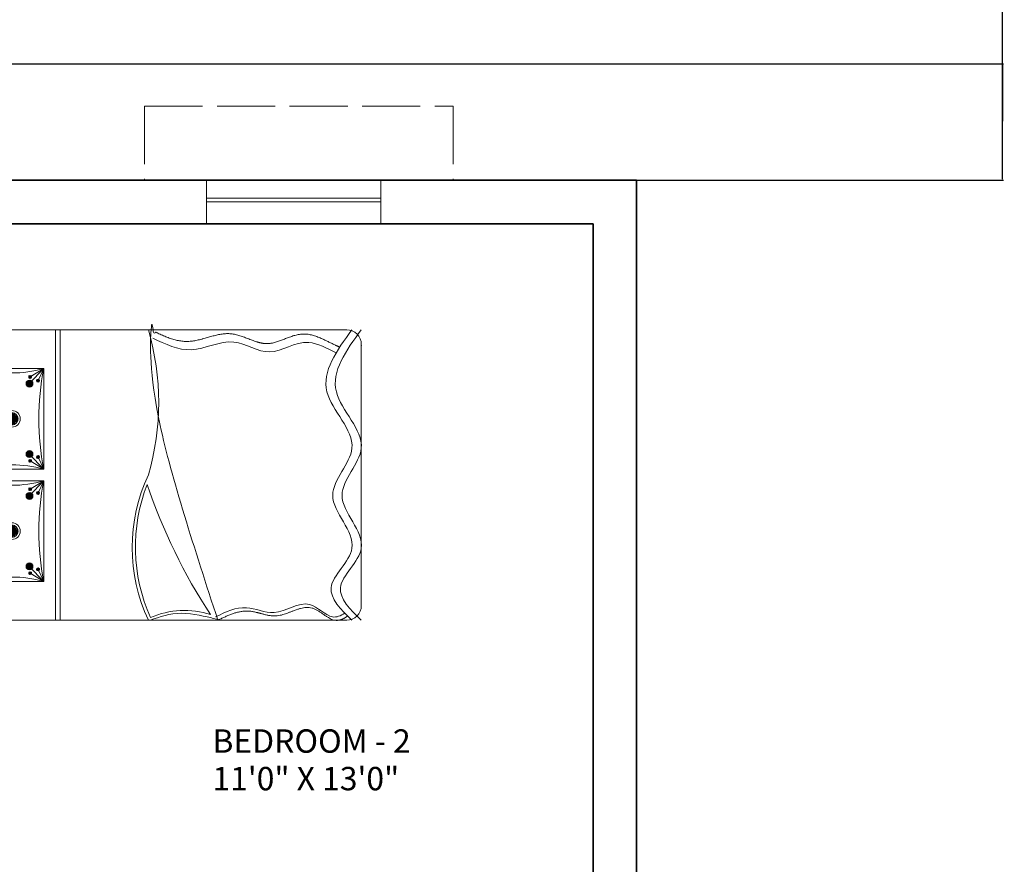
# Model space of a CAD drawing. Units: inches. Extents: x -61 to 1599, y -1316 to 257.
# Tile 182 of 204: x 1395 to 1599, y -753 to -579. Entities that reach past the tile are written whole.
import ezdxf

# ---------------------------------------------------------------- set-up
doc = ezdxf.new("R2010")
doc.units = ezdxf.units.IN
doc.header["$MEASUREMENT"] = 0
doc.linetypes.add('ACAD_ISO02W100', pattern=[15, 12, -3])
for name, color, linetype, lineweight in [('A-ANNO-DIMS', 2, 'Continuous', 18), ('A-AREA-IDEN', 1, 'Continuous', 18), ('A-FLOR-OVHD', 203, 'ACAD_ISO02W100', 13), ('FURNITURE', 83, 'Continuous', 18), ('WALLS', 4, 'Continuous', 35), ('WINDOWS', 220, 'Continuous', 18)]:
    doc.layers.add(name, color=color, linetype=linetype, lineweight=lineweight)
doc.layers.add('LT', color=8, linetype='Continuous')
doc.styles.get("Standard").update_dxf_attribs({"font": 'arial.ttf'})
doc.dimstyles.get("Standard").update_dxf_attribs({"dimtxt": 0.18, "dimasz": 0.18, "dimexe": 0.18, "dimexo": 0.0625, "dimgap": 0.09, "dimtad": 0, "dimtih": 1, "dimtoh": 1, "dimdec": 0, "dimzin": 0, "dimdsep": 46, "dimlunit": 3, "dimtxsty": 'Standard', "dimcen": 0.09, "dimadec": 0, "dimazin": 0, "dimtfac": 1, "dimtdec": 0, "dimtofl": 0, "dimtmove": 0, "dimatfit": 3, "dimfxl": 1, "dimtolj": 1, "dimtzin": 0, "dimarcsym": 0})

# ---------------------------------------------------------------- blocks, each defined once
blk = doc.blocks.new('WIN-36IN')
for p, q in [((0, 4.5), (0, 9)), ((0, 9), (0, 0)), ((36, 9), (36, 0)), ((0, 5.26), (36, 5.26)), ((0, 4.5), (36, 4.5)), ((0, 4.5), (36, 4.5))]:
    blk.add_line(p, q)
blk = doc.blocks.new('*U100')
at = {"layer": 'LT'}
blk.add_line((0, 0.15), (0, -0.15), dxfattribs=at)
for centre, start, end in [((0.44, 0), 160.9983, 199.0017), ((-0.44, 0), 340.9983, 19.0017)]:
    blk.add_arc(centre, 0.468, start, end, dxfattribs=at)
blk = doc.blocks.new('*U101')
at = {"layer": 'LT', "transparency": 16777216}
for p, rotation in [((-57.96, -16.31), 72), ((-57.93, -16.26), 48.00000000000001), ((-57.87, -16.22), 24), ((-57.75, -16.22), 336), ((-57.7, -16.26), 312), ((-57.67, -16.31), 288), ((-57.96, -16.37), 96), ((-57.94, -16.43), 120), ((-57.9, -16.48), 144), ((-57.84, -16.51), 168.0000000000001), ((-57.78, -16.51), 192), ((-57.72, -16.48), 216), ((-57.68, -16.43), 240), ((-57.66, -16.37), 264)]:
    blk.add_blockref('*U100', p, dxfattribs=dict(at, rotation=rotation))
blk.add_blockref('*U100', (-57.81, -16.21), dxfattribs=at)
blk = doc.blocks.new('*U104')
at = {"layer": 'LT'}
blk.add_line((0, 0.15), (0, -0.15), dxfattribs=at)
for centre, start, end in [((0.44, 0), 160.9983, 199.0017), ((-0.44, 0), 340.9983, 19.0017)]:
    blk.add_arc(centre, 0.468, start, end, dxfattribs=at)
blk = doc.blocks.new('*U105')
at = {"layer": 'LT', "transparency": 16777216}
for p, rotation in [((-57.96, -16.31), 72), ((-57.93, -16.26), 48.00000000000001), ((-57.87, -16.22), 24), ((-57.75, -16.22), 336), ((-57.7, -16.26), 312), ((-57.67, -16.31), 288), ((-57.96, -16.37), 96), ((-57.94, -16.43), 120), ((-57.9, -16.48), 144), ((-57.84, -16.51), 168.0000000000001), ((-57.78, -16.51), 192), ((-57.72, -16.48), 216), ((-57.68, -16.43), 240), ((-57.66, -16.37), 264)]:
    blk.add_blockref('*U104', p, dxfattribs=dict(at, rotation=rotation))
blk.add_blockref('*U104', (-57.81, -16.21), dxfattribs=at)
blk = doc.blocks.new('*U71')
at = {"layer": 'LT'}
blk.add_line((0, 0.15), (0, -0.15), dxfattribs=at)
for centre, start, end in [((0.44, 0), 160.9983, 199.0017), ((-0.44, 0), 340.9983, 19.0017)]:
    blk.add_arc(centre, 0.468, start, end, dxfattribs=at)
blk = doc.blocks.new('*U58')
at = {"layer": 'LT', "transparency": 16777216}
for p, rotation in [((-57.96, -16.31), 72), ((-57.93, -16.26), 48.00000000000001), ((-57.87, -16.22), 24), ((-57.75, -16.22), 336), ((-57.7, -16.26), 312), ((-57.67, -16.31), 288), ((-57.96, -16.37), 96), ((-57.94, -16.43), 120), ((-57.9, -16.48), 144), ((-57.84, -16.51), 168.0000000000001), ((-57.78, -16.51), 192), ((-57.72, -16.48), 216), ((-57.68, -16.43), 240), ((-57.66, -16.37), 264)]:
    blk.add_blockref('*U71', p, dxfattribs=dict(at, rotation=rotation))
blk.add_blockref('*U71', (-57.81, -16.21), dxfattribs=at)
blk = doc.blocks.new('*U61')
at = {"layer": 'LT'}
blk.add_line((0, 0.15), (0, -0.15), dxfattribs=at)
for centre, start, end in [((0.44, 0), 160.9983, 199.0017), ((-0.44, 0), 340.9983, 19.0017)]:
    blk.add_arc(centre, 0.468, start, end, dxfattribs=at)
blk = doc.blocks.new('*U62')
at = {"layer": 'LT', "transparency": 16777216}
for p, rotation in [((-57.96, -16.31), 72), ((-57.93, -16.26), 48.00000000000001), ((-57.87, -16.22), 24), ((-57.75, -16.22), 336), ((-57.7, -16.26), 312), ((-57.67, -16.31), 288), ((-57.96, -16.37), 96), ((-57.94, -16.43), 120), ((-57.9, -16.48), 144), ((-57.84, -16.51), 168.0000000000001), ((-57.78, -16.51), 192), ((-57.72, -16.48), 216), ((-57.68, -16.43), 240), ((-57.66, -16.37), 264)]:
    blk.add_blockref('*U61', p, dxfattribs=dict(at, rotation=rotation))
blk.add_blockref('*U61', (-57.81, -16.21), dxfattribs=at)
blk = doc.blocks.new('*U94')
at = {"layer": 'LT'}
blk.add_line((0, 0.36), (0, -0.36), dxfattribs=at)
for centre, start, end in [((1.04, 0), 160.9983, 199.0017), ((-1.04, 0), 340.9983, 19.0017)]:
    blk.add_arc(centre, 1.1, start, end, dxfattribs=at)
blk = doc.blocks.new('*U95')
at = {"layer": 'LT', "transparency": 16777216}
for p, rotation in [((-136.32, -38.51), 96), ((-136.3, -38.36), 72), ((-136.27, -38.65), 120), ((-136.23, -38.23), 48.00000000000001), ((-136.17, -38.76), 144), ((-136.11, -38.14), 23.99999999999999), ((-136.04, -38.82), 168.0000000000001), ((-135.82, -38.14), 336.0000000000001), ((-135.89, -38.82), 191.9999999999999), ((-135.75, -38.76), 216), ((-135.69, -38.23), 312), ((-135.65, -38.65), 240), ((-135.62, -38.36), 288.0000000000001), ((-135.6, -38.51), 264)]:
    blk.add_blockref('*U94', p, dxfattribs=dict(at, rotation=rotation))
blk.add_blockref('*U94', (-135.96, -38.11), dxfattribs=at)
blk = doc.blocks.new('*U57')
at = {"layer": 'LT'}
blk.add_line((0, 0.36), (0, -0.36), dxfattribs=at)
for centre, start, end in [((1.04, 0), 160.9983, 199.0017), ((-1.04, 0), 340.9983, 19.0017)]:
    blk.add_arc(centre, 1.1, start, end, dxfattribs=at)
blk = doc.blocks.new('*U99')
at = {"layer": 'LT', "transparency": 16777216}
for p, rotation in [((-136.32, -38.51), 96), ((-136.3, -38.36), 72), ((-136.27, -38.65), 120), ((-136.23, -38.23), 48.00000000000001), ((-136.17, -38.76), 144), ((-136.11, -38.14), 23.99999999999999), ((-136.04, -38.82), 168.0000000000001), ((-135.82, -38.14), 336.0000000000001), ((-135.89, -38.82), 191.9999999999999), ((-135.75, -38.76), 216), ((-135.69, -38.23), 312), ((-135.65, -38.65), 240), ((-135.62, -38.36), 288.0000000000001), ((-135.6, -38.51), 264)]:
    blk.add_blockref('*U57', p, dxfattribs=dict(at, rotation=rotation))
blk.add_blockref('*U57', (-135.96, -38.11), dxfattribs=at)
blk = doc.blocks.new('*U80')
at = {"layer": 'LT'}
blk.add_line((0, 0.36), (0, -0.36), dxfattribs=at)
for centre, start, end in [((1.04, 0), 160.9983, 199.0017), ((-1.04, 0), 340.9983, 19.0017)]:
    blk.add_arc(centre, 1.1, start, end, dxfattribs=at)
blk = doc.blocks.new('*U96')
at = {"layer": 'LT', "transparency": 16777216}
for p, rotation in [((-136.32, -38.51), 96), ((-136.3, -38.36), 72), ((-136.27, -38.65), 120), ((-136.23, -38.23), 48.00000000000001), ((-136.17, -38.76), 144), ((-136.11, -38.14), 23.99999999999999), ((-136.04, -38.82), 168.0000000000001), ((-135.82, -38.14), 336.0000000000001), ((-135.89, -38.82), 191.9999999999999), ((-135.75, -38.76), 216), ((-135.69, -38.23), 312), ((-135.65, -38.65), 240), ((-135.62, -38.36), 288.0000000000001), ((-135.6, -38.51), 264)]:
    blk.add_blockref('*U80', p, dxfattribs=dict(at, rotation=rotation))
blk.add_blockref('*U80', (-135.96, -38.11), dxfattribs=at)
blk = doc.blocks.new('*U69')
at = {"layer": 'LT'}
blk.add_line((0, 0.36), (0, -0.36), dxfattribs=at)
for centre, start, end in [((1.04, 0), 160.9983, 199.0017), ((-1.04, 0), 340.9983, 19.0017)]:
    blk.add_arc(centre, 1.1, start, end, dxfattribs=at)
blk = doc.blocks.new('*U70')
at = {"layer": 'LT', "transparency": 16777216}
for p, rotation in [((-136.32, -38.51), 96), ((-136.3, -38.36), 72), ((-136.27, -38.65), 120), ((-136.23, -38.23), 48.00000000000001), ((-136.17, -38.76), 144), ((-136.11, -38.14), 23.99999999999999), ((-136.04, -38.82), 168.0000000000001), ((-135.82, -38.14), 336.0000000000001), ((-135.89, -38.82), 191.9999999999999), ((-135.75, -38.76), 216), ((-135.69, -38.23), 312), ((-135.65, -38.65), 240), ((-135.62, -38.36), 288.0000000000001), ((-135.6, -38.51), 264)]:
    blk.add_blockref('*U69', p, dxfattribs=dict(at, rotation=rotation))
blk.add_blockref('*U69', (-135.96, -38.11), dxfattribs=at)
blk = doc.blocks.new('*U102')
at = {"layer": 'LT'}
blk.add_line((0, 0.15), (0, -0.15), dxfattribs=at)
for centre, start, end in [((0.44, 0), 160.9983, 199.0017), ((-0.44, 0), 340.9983, 19.0017)]:
    blk.add_arc(centre, 0.468, start, end, dxfattribs=at)
blk = doc.blocks.new('*U103')
at = {"layer": 'LT', "transparency": 16777216}
for p, rotation in [((-57.96, -16.31), 72), ((-57.93, -16.26), 48.00000000000001), ((-57.87, -16.22), 24), ((-57.75, -16.22), 336), ((-57.7, -16.26), 312), ((-57.67, -16.31), 288), ((-57.96, -16.37), 96), ((-57.94, -16.43), 120), ((-57.9, -16.48), 144), ((-57.84, -16.51), 168.0000000000001), ((-57.78, -16.51), 192), ((-57.72, -16.48), 216), ((-57.68, -16.43), 240), ((-57.66, -16.37), 264)]:
    blk.add_blockref('*U102', p, dxfattribs=dict(at, rotation=rotation))
blk.add_blockref('*U102', (-57.81, -16.21), dxfattribs=at)
blk = doc.blocks.new('*U55')
at = {"layer": 'LT'}
blk.add_line((0, 0.15), (0, -0.15), dxfattribs=at)
for centre, start, end in [((0.44, 0), 160.9983, 199.0017), ((-0.44, 0), 340.9983, 19.0017)]:
    blk.add_arc(centre, 0.468, start, end, dxfattribs=at)
blk = doc.blocks.new('*U56')
at = {"layer": 'LT', "transparency": 16777216}
for p, rotation in [((-57.96, -16.31), 72), ((-57.93, -16.26), 48.00000000000001), ((-57.87, -16.22), 24), ((-57.75, -16.22), 336), ((-57.7, -16.26), 312), ((-57.67, -16.31), 288), ((-57.96, -16.37), 96), ((-57.94, -16.43), 120), ((-57.9, -16.48), 144), ((-57.84, -16.51), 168.0000000000001), ((-57.78, -16.51), 192), ((-57.72, -16.48), 216), ((-57.68, -16.43), 240), ((-57.66, -16.37), 264)]:
    blk.add_blockref('*U55', p, dxfattribs=dict(at, rotation=rotation))
blk.add_blockref('*U55', (-57.81, -16.21), dxfattribs=at)
blk = doc.blocks.new('*U59')
at = {"layer": 'LT'}
blk.add_line((0, 0.15), (0, -0.15), dxfattribs=at)
for centre, start, end in [((0.44, 0), 160.9983, 199.0017), ((-0.44, 0), 340.9983, 19.0017)]:
    blk.add_arc(centre, 0.468, start, end, dxfattribs=at)
blk = doc.blocks.new('*U60')
at = {"layer": 'LT', "transparency": 16777216}
for p, rotation in [((-57.96, -16.31), 72), ((-57.93, -16.26), 48.00000000000001), ((-57.87, -16.22), 24), ((-57.75, -16.22), 336), ((-57.7, -16.26), 312), ((-57.67, -16.31), 288), ((-57.96, -16.37), 96), ((-57.94, -16.43), 120), ((-57.9, -16.48), 144), ((-57.84, -16.51), 168.0000000000001), ((-57.78, -16.51), 192), ((-57.72, -16.48), 216), ((-57.68, -16.43), 240), ((-57.66, -16.37), 264)]:
    blk.add_blockref('*U59', p, dxfattribs=dict(at, rotation=rotation))
blk.add_blockref('*U59', (-57.81, -16.21), dxfattribs=at)
blk = doc.blocks.new('*U67')
at = {"layer": 'LT'}
blk.add_line((0, 0.15), (0, -0.15), dxfattribs=at)
for centre, start, end in [((0.44, 0), 160.9983, 199.0017), ((-0.44, 0), 340.9983, 19.0017)]:
    blk.add_arc(centre, 0.468, start, end, dxfattribs=at)
blk = doc.blocks.new('*U68')
at = {"layer": 'LT', "transparency": 16777216}
for p, rotation in [((-57.96, -16.31), 72), ((-57.93, -16.26), 48.00000000000001), ((-57.87, -16.22), 24), ((-57.75, -16.22), 336), ((-57.7, -16.26), 312), ((-57.67, -16.31), 288), ((-57.96, -16.37), 96), ((-57.94, -16.43), 120), ((-57.9, -16.48), 144), ((-57.84, -16.51), 168.0000000000001), ((-57.78, -16.51), 192), ((-57.72, -16.48), 216), ((-57.68, -16.43), 240), ((-57.66, -16.37), 264)]:
    blk.add_blockref('*U67', p, dxfattribs=dict(at, rotation=rotation))
blk.add_blockref('*U67', (-57.81, -16.21), dxfattribs=at)
blk = doc.blocks.new('*U106')
at = {"layer": 'LT'}
blk.add_line((0, 0.64), (0, -0.64), dxfattribs=at)
for centre, start, end in [((1.87, 0), 160.9983, 199.0017), ((-1.87, 0), 340.9983, 19.0017)]:
    blk.add_arc(centre, 1.97, start, end, dxfattribs=at)
blk = doc.blocks.new('*U93')
at = {"layer": 'LT', "transparency": 16777216}
for p, rotation in [((-244.36, -69.03), 96), ((-244.33, -68.76), 72), ((-244.28, -69.28), 120), ((-244.2, -68.53), 48.00000000000001), ((-244.1, -69.48), 144), ((-243.98, -68.38), 23.99999999999999), ((-243.86, -69.59), 168), ((-243.59, -69.59), 192), ((-243.46, -68.38), 336.0000000000001), ((-243.34, -69.48), 216), ((-243.25, -68.53), 312), ((-243.17, -69.28), 240), ((-243.11, -68.76), 288), ((-243.08, -69.03), 264)]:
    blk.add_blockref('*U106', p, dxfattribs=dict(at, rotation=rotation))
blk.add_blockref('*U106', (-243.72, -68.32), dxfattribs=at)
blk = doc.blocks.new('*U63')
at = {"layer": 'LT'}
blk.add_line((0, 0.64), (0, -0.64), dxfattribs=at)
for centre, start, end in [((1.87, 0), 160.9983, 199.0017), ((-1.87, 0), 340.9983, 19.0017)]:
    blk.add_arc(centre, 1.97, start, end, dxfattribs=at)
blk = doc.blocks.new('*U64')
at = {"layer": 'LT', "transparency": 16777216}
for p, rotation in [((-244.36, -69.03), 96), ((-244.33, -68.76), 72), ((-244.28, -69.28), 120), ((-244.2, -68.53), 48.00000000000001), ((-244.1, -69.48), 144), ((-243.98, -68.38), 23.99999999999999), ((-243.86, -69.59), 168), ((-243.59, -69.59), 192), ((-243.46, -68.38), 336.0000000000001), ((-243.34, -69.48), 216), ((-243.25, -68.53), 312), ((-243.17, -69.28), 240), ((-243.11, -68.76), 288), ((-243.08, -69.03), 264)]:
    blk.add_blockref('*U63', p, dxfattribs=dict(at, rotation=rotation))
blk.add_blockref('*U63', (-243.72, -68.32), dxfattribs=at)
blk = doc.blocks.new('*U83')
at = {"layer": 'LT'}
blk.add_line((0, 0.36), (0, -0.36), dxfattribs=at)
for centre, start, end in [((1.04, 0), 160.9983, 199.0017), ((-1.04, 0), 340.9983, 19.0017)]:
    blk.add_arc(centre, 1.1, start, end, dxfattribs=at)
blk = doc.blocks.new('*U84')
at = {"layer": 'LT', "transparency": 16777216}
for p, rotation in [((-136.32, -38.51), 96), ((-136.3, -38.36), 72), ((-136.27, -38.65), 120), ((-136.23, -38.23), 48.00000000000001), ((-136.17, -38.76), 144), ((-136.11, -38.14), 23.99999999999999), ((-136.04, -38.82), 168.0000000000001), ((-135.82, -38.14), 336.0000000000001), ((-135.89, -38.82), 191.9999999999999), ((-135.75, -38.76), 216), ((-135.69, -38.23), 312), ((-135.65, -38.65), 240), ((-135.62, -38.36), 288.0000000000001), ((-135.6, -38.51), 264)]:
    blk.add_blockref('*U83', p, dxfattribs=dict(at, rotation=rotation))
blk.add_blockref('*U83', (-135.96, -38.11), dxfattribs=at)
blk = doc.blocks.new('*U74')
at = {"layer": 'LT'}
blk.add_line((0, 0.36), (0, -0.36), dxfattribs=at)
for centre, start, end in [((1.04, 0), 160.9983, 199.0017), ((-1.04, 0), 340.9983, 19.0017)]:
    blk.add_arc(centre, 1.1, start, end, dxfattribs=at)
blk = doc.blocks.new('*U75')
at = {"layer": 'LT', "transparency": 16777216}
for p, rotation in [((-136.32, -38.51), 96), ((-136.3, -38.36), 72), ((-136.27, -38.65), 120), ((-136.23, -38.23), 48.00000000000001), ((-136.17, -38.76), 144), ((-136.11, -38.14), 23.99999999999999), ((-136.04, -38.82), 168.0000000000001), ((-135.82, -38.14), 336.0000000000001), ((-135.89, -38.82), 191.9999999999999), ((-135.75, -38.76), 216), ((-135.69, -38.23), 312), ((-135.65, -38.65), 240), ((-135.62, -38.36), 288.0000000000001), ((-135.6, -38.51), 264)]:
    blk.add_blockref('*U74', p, dxfattribs=dict(at, rotation=rotation))
blk.add_blockref('*U74', (-135.96, -38.11), dxfattribs=at)
blk = doc.blocks.new('*U65')
at = {"layer": 'LT'}
blk.add_line((0, 0.36), (0, -0.36), dxfattribs=at)
for centre, start, end in [((1.04, 0), 160.9983, 199.0017), ((-1.04, 0), 340.9983, 19.0017)]:
    blk.add_arc(centre, 1.1, start, end, dxfattribs=at)
blk = doc.blocks.new('*U66')
at = {"layer": 'LT', "transparency": 16777216}
for p, rotation in [((-136.32, -38.51), 96), ((-136.3, -38.36), 72), ((-136.27, -38.65), 120), ((-136.23, -38.23), 48.00000000000001), ((-136.17, -38.76), 144), ((-136.11, -38.14), 23.99999999999999), ((-136.04, -38.82), 168.0000000000001), ((-135.82, -38.14), 336.0000000000001), ((-135.89, -38.82), 191.9999999999999), ((-135.75, -38.76), 216), ((-135.69, -38.23), 312), ((-135.65, -38.65), 240), ((-135.62, -38.36), 288.0000000000001), ((-135.6, -38.51), 264)]:
    blk.add_blockref('*U65', p, dxfattribs=dict(at, rotation=rotation))
blk.add_blockref('*U65', (-135.96, -38.11), dxfattribs=at)
blk = doc.blocks.new('*U85')
at = {"layer": 'LT'}
blk.add_line((0, 0.36), (0, -0.36), dxfattribs=at)
for centre, start, end in [((1.04, 0), 160.9983, 199.0017), ((-1.04, 0), 340.9983, 19.0017)]:
    blk.add_arc(centre, 1.1, start, end, dxfattribs=at)
blk = doc.blocks.new('*U86')
at = {"layer": 'LT', "transparency": 16777216}
for p, rotation in [((-136.32, -38.51), 96), ((-136.3, -38.36), 72), ((-136.27, -38.65), 120), ((-136.23, -38.23), 48.00000000000001), ((-136.17, -38.76), 144), ((-136.11, -38.14), 23.99999999999999), ((-136.04, -38.82), 168.0000000000001), ((-135.82, -38.14), 336.0000000000001), ((-135.89, -38.82), 191.9999999999999), ((-135.75, -38.76), 216), ((-135.69, -38.23), 312), ((-135.65, -38.65), 240), ((-135.62, -38.36), 288.0000000000001), ((-135.6, -38.51), 264)]:
    blk.add_blockref('*U85', p, dxfattribs=dict(at, rotation=rotation))
blk.add_blockref('*U85', (-135.96, -38.11), dxfattribs=at)
blk = doc.blocks.new('*U78')
at = {"layer": 'LT'}
blk.add_line((0, 0.15), (0, -0.15), dxfattribs=at)
for centre, start, end in [((0.44, 0), 160.9983, 199.0017), ((-0.44, 0), 340.9983, 19.0017)]:
    blk.add_arc(centre, 0.468, start, end, dxfattribs=at)
blk = doc.blocks.new('*U79')
at = {"layer": 'LT', "transparency": 16777216}
for p, rotation in [((-57.96, -16.31), 72), ((-57.93, -16.26), 48.00000000000001), ((-57.87, -16.22), 24), ((-57.75, -16.22), 336), ((-57.7, -16.26), 312), ((-57.67, -16.31), 288), ((-57.96, -16.37), 96), ((-57.94, -16.43), 120), ((-57.9, -16.48), 144), ((-57.84, -16.51), 168.0000000000001), ((-57.78, -16.51), 192), ((-57.72, -16.48), 216), ((-57.68, -16.43), 240), ((-57.66, -16.37), 264)]:
    blk.add_blockref('*U78', p, dxfattribs=dict(at, rotation=rotation))
blk.add_blockref('*U78', (-57.81, -16.21), dxfattribs=at)
blk = doc.blocks.new('*U72')
at = {"layer": 'LT'}
blk.add_line((0, 0.15), (0, -0.15), dxfattribs=at)
for centre, start, end in [((0.44, 0), 160.9983, 199.0017), ((-0.44, 0), 340.9983, 19.0017)]:
    blk.add_arc(centre, 0.468, start, end, dxfattribs=at)
blk = doc.blocks.new('*U73')
at = {"layer": 'LT', "transparency": 16777216}
for p, rotation in [((-57.96, -16.31), 72), ((-57.93, -16.26), 48.00000000000001), ((-57.87, -16.22), 24), ((-57.75, -16.22), 336), ((-57.7, -16.26), 312), ((-57.67, -16.31), 288), ((-57.96, -16.37), 96), ((-57.94, -16.43), 120), ((-57.9, -16.48), 144), ((-57.84, -16.51), 168.0000000000001), ((-57.78, -16.51), 192), ((-57.72, -16.48), 216), ((-57.68, -16.43), 240), ((-57.66, -16.37), 264)]:
    blk.add_blockref('*U72', p, dxfattribs=dict(at, rotation=rotation))
blk.add_blockref('*U72', (-57.81, -16.21), dxfattribs=at)
blk = doc.blocks.new('*U89')
at = {"layer": 'LT'}
blk.add_line((0, 0.15), (0, -0.15), dxfattribs=at)
for centre, start, end in [((0.44, 0), 160.9983, 199.0017), ((-0.44, 0), 340.9983, 19.0017)]:
    blk.add_arc(centre, 0.468, start, end, dxfattribs=at)
blk = doc.blocks.new('*U90')
at = {"layer": 'LT', "transparency": 16777216}
for p, rotation in [((-57.96, -16.31), 72), ((-57.93, -16.26), 48.00000000000001), ((-57.87, -16.22), 24), ((-57.75, -16.22), 336), ((-57.7, -16.26), 312), ((-57.67, -16.31), 288), ((-57.96, -16.37), 96), ((-57.94, -16.43), 120), ((-57.9, -16.48), 144), ((-57.84, -16.51), 168.0000000000001), ((-57.78, -16.51), 192), ((-57.72, -16.48), 216), ((-57.68, -16.43), 240), ((-57.66, -16.37), 264)]:
    blk.add_blockref('*U89', p, dxfattribs=dict(at, rotation=rotation))
blk.add_blockref('*U89', (-57.81, -16.21), dxfattribs=at)
blk = doc.blocks.new('*U97')
at = {"layer": 'LT'}
blk.add_line((0, 0.15), (0, -0.15), dxfattribs=at)
for centre, start, end in [((0.44, 0), 160.9983, 199.0017), ((-0.44, 0), 340.9983, 19.0017)]:
    blk.add_arc(centre, 0.468, start, end, dxfattribs=at)
blk = doc.blocks.new('*U98')
at = {"layer": 'LT', "transparency": 16777216}
for p, rotation in [((-57.96, -16.31), 72), ((-57.93, -16.26), 48.00000000000001), ((-57.87, -16.22), 24), ((-57.75, -16.22), 336), ((-57.7, -16.26), 312), ((-57.67, -16.31), 288), ((-57.96, -16.37), 96), ((-57.94, -16.43), 120), ((-57.9, -16.48), 144), ((-57.84, -16.51), 168.0000000000001), ((-57.78, -16.51), 192), ((-57.72, -16.48), 216), ((-57.68, -16.43), 240), ((-57.66, -16.37), 264)]:
    blk.add_blockref('*U97', p, dxfattribs=dict(at, rotation=rotation))
blk.add_blockref('*U97', (-57.81, -16.21), dxfattribs=at)
blk = doc.blocks.new('*U76')
at = {"layer": 'LT'}
blk.add_line((0, 0.15), (0, -0.15), dxfattribs=at)
for centre, start, end in [((0.44, 0), 160.9983, 199.0017), ((-0.44, 0), 340.9983, 19.0017)]:
    blk.add_arc(centre, 0.468, start, end, dxfattribs=at)
blk = doc.blocks.new('*U77')
at = {"layer": 'LT', "transparency": 16777216}
for p, rotation in [((-57.96, -16.31), 72), ((-57.93, -16.26), 48.00000000000001), ((-57.87, -16.22), 24), ((-57.75, -16.22), 336), ((-57.7, -16.26), 312), ((-57.67, -16.31), 288), ((-57.96, -16.37), 96), ((-57.94, -16.43), 120), ((-57.9, -16.48), 144), ((-57.84, -16.51), 168.0000000000001), ((-57.78, -16.51), 192), ((-57.72, -16.48), 216), ((-57.68, -16.43), 240), ((-57.66, -16.37), 264)]:
    blk.add_blockref('*U76', p, dxfattribs=dict(at, rotation=rotation))
blk.add_blockref('*U76', (-57.81, -16.21), dxfattribs=at)
blk = doc.blocks.new('*U81')
at = {"layer": 'LT'}
blk.add_line((0, 0.15), (0, -0.15), dxfattribs=at)
for centre, start, end in [((0.44, 0), 160.9983, 199.0017), ((-0.44, 0), 340.9983, 19.0017)]:
    blk.add_arc(centre, 0.468, start, end, dxfattribs=at)
blk = doc.blocks.new('*U82')
at = {"layer": 'LT', "transparency": 16777216}
for p, rotation in [((-57.96, -16.31), 72), ((-57.93, -16.26), 48.00000000000001), ((-57.87, -16.22), 24), ((-57.75, -16.22), 336), ((-57.7, -16.26), 312), ((-57.67, -16.31), 288), ((-57.96, -16.37), 96), ((-57.94, -16.43), 120), ((-57.9, -16.48), 144), ((-57.84, -16.51), 168.0000000000001), ((-57.78, -16.51), 192), ((-57.72, -16.48), 216), ((-57.68, -16.43), 240), ((-57.66, -16.37), 264)]:
    blk.add_blockref('*U81', p, dxfattribs=dict(at, rotation=rotation))
blk.add_blockref('*U81', (-57.81, -16.21), dxfattribs=at)
blk = doc.blocks.new('*U87')
at = {"layer": 'LT'}
blk.add_line((0, 0.15), (0, -0.15), dxfattribs=at)
for centre, start, end in [((0.44, 0), 160.9983, 199.0017), ((-0.44, 0), 340.9983, 19.0017)]:
    blk.add_arc(centre, 0.468, start, end, dxfattribs=at)
blk = doc.blocks.new('*U88')
at = {"layer": 'LT', "transparency": 16777216}
for p, rotation in [((-57.96, -16.31), 72), ((-57.93, -16.26), 48.00000000000001), ((-57.87, -16.22), 24), ((-57.75, -16.22), 336), ((-57.7, -16.26), 312), ((-57.67, -16.31), 288), ((-57.96, -16.37), 96), ((-57.94, -16.43), 120), ((-57.9, -16.48), 144), ((-57.84, -16.51), 168.0000000000001), ((-57.78, -16.51), 192), ((-57.72, -16.48), 216), ((-57.68, -16.43), 240), ((-57.66, -16.37), 264)]:
    blk.add_blockref('*U87', p, dxfattribs=dict(at, rotation=rotation))
blk.add_blockref('*U87', (-57.81, -16.21), dxfattribs=at)
blk = doc.blocks.new('*U91')
at = {"layer": 'LT'}
blk.add_line((0, 0.15), (0, -0.15), dxfattribs=at)
for centre, start, end in [((0.44, 0), 160.9983, 199.0017), ((-0.44, 0), 340.9983, 19.0017)]:
    blk.add_arc(centre, 0.468, start, end, dxfattribs=at)
blk = doc.blocks.new('*U92')
at = {"layer": 'LT', "transparency": 16777216}
for p, rotation in [((-57.96, -16.31), 72), ((-57.93, -16.26), 48.00000000000001), ((-57.87, -16.22), 24), ((-57.75, -16.22), 336), ((-57.7, -16.26), 312), ((-57.67, -16.31), 288), ((-57.96, -16.37), 96), ((-57.94, -16.43), 120), ((-57.9, -16.48), 144), ((-57.84, -16.51), 168.0000000000001), ((-57.78, -16.51), 192), ((-57.72, -16.48), 216), ((-57.68, -16.43), 240), ((-57.66, -16.37), 264)]:
    blk.add_blockref('*U91', p, dxfattribs=dict(at, rotation=rotation))
blk.add_blockref('*U91', (-57.81, -16.21), dxfattribs=at)
blk = doc.blocks.new('BED-DOUBLE-COMPACT')
for p, q in [((16.8, 60.04), (16.8, 0.04)), ((17.8, 60.04), (17.8, 0.04)), ((1.2, 52.04), (14.4, 52.04)), ((1.2, 52.04), (2.4, 49.53)), ((1.2, 52.04), (4.2, 48.93)), ((1.2, 52.04), (4.03, 50.31)), ((14.4, 52.04), (11.4, 48.93)), ((14.4, 52.04), (11.57, 50.31)), ((14.4, 52.04), (13.2, 49.53)), ((14.4, 31.24), (14.4, 52.04)), ((2.4, 49.53), (2.7, 49.53)), ((4.03, 50.31), (4.33, 50.31)), ((4.16, 48.92), (4.88, 48.92)), ((11.44, 48.92), (10.72, 48.92)), ((11.57, 50.31), (11.27, 50.31)), ((13.2, 49.53), (12.9, 49.53)), ((7.8, 41.64), (9.09, 41.64)), ((1.2, 31.24), (4.2, 34.34)), ((1.2, 31.24), (2.4, 33.74)), ((1.2, 31.24), (4.03, 32.96)), ((2.4, 33.74), (2.7, 33.74)), ((4.03, 32.96), (4.33, 32.96)), ((4.16, 34.35), (4.88, 34.35)), ((11.44, 34.35), (10.72, 34.35)), ((11.57, 32.96), (11.27, 32.96)), ((14.4, 31.24), (11.4, 34.34)), ((14.4, 31.24), (11.57, 32.96)), ((13.2, 33.74), (12.9, 33.74)), ((14.4, 31.24), (13.2, 33.74)), ((1.2, 31.24), (1.2, 31.24)), ((1.2, 28.84), (14.4, 28.84)), ((1.2, 28.84), (2.4, 26.33)), ((1.2, 28.84), (4.2, 25.73)), ((1.2, 28.84), (4.03, 27.11)), ((14.4, 28.84), (11.4, 25.73)), ((14.4, 28.84), (11.57, 27.11)), ((14.4, 28.84), (13.2, 26.33)), ((14.4, 8.04), (14.4, 28.84)), ((4.03, 27.11), (4.33, 27.11)), ((11.57, 27.11), (11.27, 27.11)), ((2.4, 26.33), (2.7, 26.33)), ((4.16, 25.72), (4.88, 25.72)), ((11.44, 25.72), (10.72, 25.72)), ((13.2, 26.33), (12.9, 26.33)), ((7.8, 18.44), (9.09, 18.44)), ((1.2, 8.04), (4.2, 11.14)), ((1.2, 8.04), (2.4, 10.54)), ((2.4, 10.54), (2.7, 10.54)), ((4.16, 11.15), (4.88, 11.15)), ((11.44, 11.15), (10.72, 11.15)), ((14.4, 8.04), (11.4, 11.14)), ((13.2, 10.54), (12.9, 10.54)), ((14.4, 8.04), (13.2, 10.54)), ((1.2, 8.04), (4.03, 9.76)), ((4.03, 9.76), (4.33, 9.76)), ((11.57, 9.76), (11.27, 9.76)), ((14.4, 8.04), (11.57, 9.76)), ((1.2, 8.04), (1.2, 8.04))]:
    blk.add_line(p, q)
for points in [[(77, 60.04), (3, 60.04, 0.414214), (0, 57.04), (0, 3.04, 0.414214), (3, 0.04), (77, 0.04, 0.414214), (80, 3.04), (80, 57.04, 0.414214)], [(2.7, 49.53, 0.167358), (2.4, 49.53, 0.167358)], [(4.33, 50.31, 0.167358), (4.03, 50.31, 0.167358)], [(4.88, 48.92, 0.167358), (4.16, 48.92, 0.167358)], [(11.44, 48.92, 0.167358), (10.72, 48.92, 0.167358)], [(11.57, 50.31, 0.167358), (11.27, 50.31, 0.167358)], [(13.2, 49.53, 0.167358), (12.9, 49.53, 0.167358)], [(7.8, 41.64, 0.167358), (9.09, 41.64, 0.167358)], [(2.4, 33.74, 0.167358), (2.7, 33.74, 0.167358)], [(4.03, 32.96, 0.167358), (4.33, 32.96, 0.167358)], [(4.16, 34.35, 0.167358), (4.88, 34.35, 0.167358)], [(10.72, 34.35, 0.167358), (11.44, 34.35, 0.167358)], [(11.27, 32.96, 0.167358), (11.57, 32.96, 0.167358)], [(4.33, 27.11, 0.167358), (4.03, 27.11, 0.167358)], [(11.57, 27.11, 0.167358), (11.27, 27.11, 0.167358)], [(35.77, 28.09, 0.064396), (48.86, 1.19, 0.181766), (36.45, 0.6, -0.202767)], [(2.7, 26.33, 0.167358), (2.4, 26.33, 0.167358)], [(4.88, 25.72, 0.167358), (4.16, 25.72, 0.167358)], [(11.44, 25.72, 0.167358), (10.72, 25.72, 0.167358)], [(13.2, 26.33, 0.167358), (12.9, 26.33, 0.167358)], [(7.8, 18.44, 0.167358), (9.09, 18.44, 0.167358)], [(2.4, 10.54, 0.167358), (2.7, 10.54, 0.167358)], [(4.16, 11.15, 0.167358), (4.88, 11.15, 0.167358)], [(10.72, 11.15, 0.167358), (11.44, 11.15, 0.167358)], [(4.03, 9.76, 0.167358), (4.33, 9.76, 0.167358)], [(11.27, 9.76, 0.167358), (11.57, 9.76, 0.167358)]]:
    blk.add_lwpolyline(points, format="xyb", close=True)
blk.add_lwpolyline([(36, 0.04, -0.22309), (36, 30.04, 0.142156), (36, 60.04)], format="xyb")
for points in [[(14.4, 31.24), (1.2, 31.24), (1.2, 52.04), (14.4, 52.04), (14.4, 31.24), (1.2, 31.24), (1.2, 52.04)], [(14.4, 8.04), (1.2, 8.04), (1.2, 28.84)]]:
    blk.add_lwpolyline(points)
for centre, radius in [((2.4, 49.53), 0.305), ((4.16, 48.92), 0.717), ((4.03, 50.31), 0.305), ((11.44, 48.92), 0.717), ((11.57, 50.31), 0.305), ((13.2, 49.53), 0.305), ((7.8, 41.64), 1.72), ((7.8, 41.64), 1.29), ((4.16, 34.35), 0.717), ((11.44, 34.35), 0.717), ((2.4, 33.74), 0.305), ((4.03, 32.96), 0.305), ((11.57, 32.96), 0.305), ((13.2, 33.74), 0.305), ((2.4, 26.33), 0.305), ((4.03, 27.11), 0.305), ((11.57, 27.11), 0.305), ((13.2, 26.33), 0.305), ((4.16, 25.72), 0.717), ((11.44, 25.72), 0.717), ((7.8, 18.44), 1.72), ((7.8, 18.44), 1.29), ((2.4, 10.54), 0.305), ((4.16, 11.15), 0.717), ((11.44, 11.15), 0.717), ((13.2, 10.54), 0.305), ((4.03, 9.76), 0.305), ((11.57, 9.76), 0.305)]:
    blk.add_circle(centre, radius)
for centre, radius, start, end in [((-49.23, 41.64), 51.49, 348.3468, 11.6532), ((7.8, 75.06), 23.95, 254.0046, 285.9954), ((64.83, 41.64), 51.49, 168.3468, 191.6532), ((13.05, 33.3), 0.468, 70.9983, 109.0017), ((13.05, 34.18), 0.468, 250.9983, 289.0017), ((7.8, 8.21), 23.95, 74.0046, 105.9954), ((-49.23, 18.44), 51.49, 348.3468, 11.6532), ((7.8, 51.86), 23.95, 254.0046, 285.9954), ((64.83, 18.44), 51.49, 168.3468, 191.6532), ((13.05, 10.1), 0.468, 70.9983, 109.0017), ((13.05, 10.98), 0.468, 250.9983, 289.0017), ((7.8, -14.99), 23.95, 74.0046, 105.9954)]:
    blk.add_arc(centre, radius, start, end)
for points, weights, knots in [([(50.36, 0.04), (44.31, 9.08), (39.57, 18.88), (36.25, 29.24), (36.33, 29.43), (36.41, 29.62), (36.5, 29.81), (39.38, 39.75), (39.36, 50.11), (36.43, 60.04), (39.05, 58.77), (44.5, 56.15), (52.79, 61.02), (60.85, 55.2), (67.65, 61.05), (73.39, 57.36), (75.56, 56.45)], [1, 0.993520320424, 0.993520320424, 1, 0.99997444972, 0.99997444972, 1, 0.973174868659, 0.973174868659, 1, 1, 1, 1, 1, 1, 1, 1], [0, 0, 0, 0, 0.279074, 0.279074, 0.279074, 0.296584, 0.296584, 0.296584, 0.865868, 0.865868, 0.865868, 9.142578, 18.107734, 25.769226, 34.110801, 40.441511, 40.441511, 40.441511, 40.441511]), ([(36.38, 0.04), (40.9, 1.99), (45.83, 1.99), (50.36, 0.04), (52.47, 1.05), (56.42, 2.94), (63, -0.48), (69.27, 4.67), (73.92, -0.77), (76.3, 0.25), (77.18, 0.91)], [1, 0.945466318698, 0.945466318698, 1, 1, 1, 1, 1, 1, 1, 1], [0, 0, 0, 0, 0.814571, 0.814571, 0.814571, 7.464247, 13.266353, 20.788537, 26.138745, 29.321895, 29.321895, 29.321895, 29.321895])]:
    blk.add_rational_spline(points, weights, degree=3, knots=knots)
for points, knots in [([(78.07, 0.04), (75.8, 2.26), (70.92, 7.04), (82.19, 15.5), (70.03, 25.56), (82.2, 36.26), (68.97, 47.49), (74.96, 55.75), (78.07, 60.04)], [0, 0, 0, 0, 7.980285, 17.179806, 28.830278, 39.318084, 52.078264, 65.891546, 65.891546, 65.891546, 65.891546]), ([(80, 0.04), (77.73, 2.26), (72.85, 7.04), (84.12, 15.5), (71.96, 25.56), (84.13, 36.26), (70.9, 47.49), (76.89, 55.75), (80, 60.04)], [0, 0, 0, 0, 7.980285, 17.179806, 28.830278, 39.318084, 52.078264, 65.891546, 65.891546, 65.891546, 65.891546]), ([(36.91, 58.31), (39.53, 57.05), (44.98, 54.43), (53.27, 59.3), (61.33, 53.48), (67.78, 59.03), (72.97, 56.17), (74.83, 55.28)], [0, 0, 0, 0, 8.27671, 17.241866, 24.903358, 33.244933, 38.427294, 38.427294, 38.427294, 38.427294]), ([(49.89, 0.74), (52, 1.75), (55.95, 3.65), (62.54, 0.23), (68.8, 5.38), (73.4, -0.01), (75.74, 0.92), (76.58, 1.52)], [0, 0, 0, 0, 6.649676, 12.451782, 19.973966, 25.324174, 28.349676, 28.349676, 28.349676, 28.349676])]:
    blk.add_open_spline(points, degree=3, knots=knots)
blk.add_open_spline([(80, 56.78), (80.02, 56.81), (80.03, 56.83), (80.05, 56.85)], degree=3)
at = {"xscale": -1}
for name, p, rotation in [('*U62', (-13.96, -8.28), 90), ('*U70', (-34.31, -87.04), 90), ('*U68', (-12.33, -7.5), 90), ('*U66', (49.91, 170.31), 270), ('*U90', (27.93, 90.77), 270), ('*U88', (29.56, 91.55), 270), ('*U105', (-13.96, -31.48), 90), ('*U56', (-12.33, -30.7), 90), ('*U99', (-34.31, -110.24), 90), ('*U84', (49.91, 147.11), 270), ('*U77', (29.56, 68.35), 270), ('*U79', (27.93, 67.57), 270)]:
    blk.add_blockref(name, p, dxfattribs=dict(at, rotation=rotation))
for name, p, rotation in [('*U86', (49.91, -87.04), 270), ('*U98', (27.93, -7.5), 270), ('*U92', (29.56, -8.28), 270), ('*U64', (-61.16, 285.36), 89.99999999999999), ('*U96', (-34.31, 170.31), 89.99999999999999), ('*U58', (-13.96, 91.55), 89.99999999999999), ('*U60', (-12.33, 90.77), 89.99999999999999), ('*U73', (27.93, -30.7), 270), ('*U82', (29.56, -31.48), 270), ('*U75', (49.91, -110.24), 270), ('*U93', (-61.16, 262.16), 89.99999999999999), ('*U101', (-13.96, 68.35), 89.99999999999999), ('*U95', (-34.31, 147.11), 89.99999999999999), ('*U103', (-12.33, 67.57), 89.99999999999999)]:
    blk.add_blockref(name, p, dxfattribs=dict(rotation=rotation))
blk = doc.blocks.new('*D694')
at = {"layer": 'A-ANNO-DIMS', "color": 0, "lineweight": -2, "transparency": 16777216}
for p, q in [((1522.77, -441.32), (1598.48, -441.32)), ((1598.3, -441.5), (1598.3, -526.56)), ((1598.3, -611.99), (1598.3, -526.93)), ((1522.77, -612.17), (1598.48, -612.17))]:
    blk.add_line(p, q, dxfattribs=at)
at = {"layer": 'A-ANNO-DIMS', "color": 0, "transparency": 16777216}
for points in [[(1598.27, -441.5), (1598.33, -441.5), (1598.3, -441.32)], [(1598.27, -611.99), (1598.33, -611.99), (1598.3, -612.17)]]:
    blk.add_solid(points, dxfattribs=at)
at = {"layer": 'DEFPOINTS', "color": 0, "transparency": 16777216}
for p in [(1522.7, -441.32), (1598.3, -441.32), (1522.7, -612.17)]:
    blk.add_point(p, dxfattribs=at)
at = {"layer": 'A-ANNO-DIMS', "color": 0, "transparency": 16777216, "insert": (1598.3, -526.75), "char_height": 0.18, "attachment_point": 5}
blk.add_mtext('\\A1;170.85', dxfattribs=at)
blk = doc.blocks.new('*D709')
at = {"layer": 'A-ANNO-DIMS', "color": 0, "lineweight": -2, "transparency": 16777216}
for p, q in [((1381.77, -588.17), (1598.48, -588.17)), ((1598.3, -588.35), (1598.3, -599.99)), ((1598.3, -611.99), (1598.3, -600.35)), ((1381.77, -612.17), (1598.48, -612.17))]:
    blk.add_line(p, q, dxfattribs=at)
at = {"layer": 'A-ANNO-DIMS', "color": 0, "transparency": 16777216}
for points in [[(1598.27, -588.35), (1598.33, -588.35), (1598.3, -588.17)], [(1598.27, -611.99), (1598.33, -611.99), (1598.3, -612.17)]]:
    blk.add_solid(points, dxfattribs=at)
at = {"layer": 'DEFPOINTS', "color": 0, "transparency": 16777216}
for p in [(1381.7, -588.17), (1381.7, -612.17), (1598.3, -612.17)]:
    blk.add_point(p, dxfattribs=at)
at = {"layer": 'A-ANNO-DIMS', "color": 0, "transparency": 16777216, "insert": (1598.3, -600.17), "char_height": 0.18, "attachment_point": 5}
blk.add_mtext('\\A1;24', dxfattribs=at)

msp = doc.modelspace()

# ---------------------------------------------------------------- linework, layer by layer
at = {"layer": 'A-FLOR-OVHD'}
for p, q in [((1420.9886, -596.8766), (1420.9886, -612.169)), ((1420.9886, -596.8766), (1484.76, -596.8766)), ((1484.76, -596.8766), (1484.76, -612.169))]:
    msp.add_line(p, q, dxfattribs=at)
at = {"layer": 'WALLS'}
for p, q in [((1522.7028, -612.169), (992.7028, -612.169)), ((1522.7028, -612.169), (1522.7028, -735.0151)), ((1381.7028, -621.169), (1513.7028, -621.169)), ((1513.7028, -621.169), (1513.7028, -777.169)), ((1522.7028, -830.3954), (1522.7028, -735.0151))]:
    msp.add_line(p, q, dxfattribs=at)

# ---------------------------------------------------------------- block references
at = {"layer": 'FURNITURE'}
msp.add_blockref('BED-DOUBLE-COMPACT', (1385.794, -703.1131), dxfattribs=at)
at = {"layer": 'WINDOWS'}
msp.add_blockref('WIN-36IN', (1433.8326, -621.1691), dxfattribs=at)

# ---------------------------------------------------------------- texts
at = {"layer": 'A-AREA-IDEN'}
for s, p in [('BEDROOM - 2', (1435.0332, -730.4455)), ('11\'0" X 13\'0"', (1435.0332, -738.2078))]:
    msp.add_text(s, height=4.832098, dxfattribs=at).set_placement(p)

# ---------------------------------------------------------------- dimensions: what is measured, and where the dimension line sits
at = {"layer": 'A-ANNO-DIMS'}
for base, p1, p2, override, picture, middle in [((1598.3028, -441.3229), (1522.7028, -612.169), (1522.7028, -441.3229), {"dimdec": 2, "dimlfac": 1, "dimrnd": 0, "dimzin": 0, "dimdsep": 46, "dimlunit": 2}, '*D694', (1598.3028, -526.746)), ((1598.3028, -612.169), (1381.7028, -588.169), (1381.7028, -612.169), {"dimdec": 0, "dimlfac": 1, "dimrnd": 0, "dimzin": 0, "dimdsep": 46, "dimlunit": 2}, '*D709', (1598.3028, -600.169))]:
    dim = msp.add_linear_dim(base=base, p1=p1, p2=p2, angle=90, dimstyle='Standard', override=override, dxfattribs=at)
    dim.commit()
    dim.dimension.update_dxf_attribs({"geometry": picture, "text_midpoint": middle})

doc.saveas('drawing.dxf')
